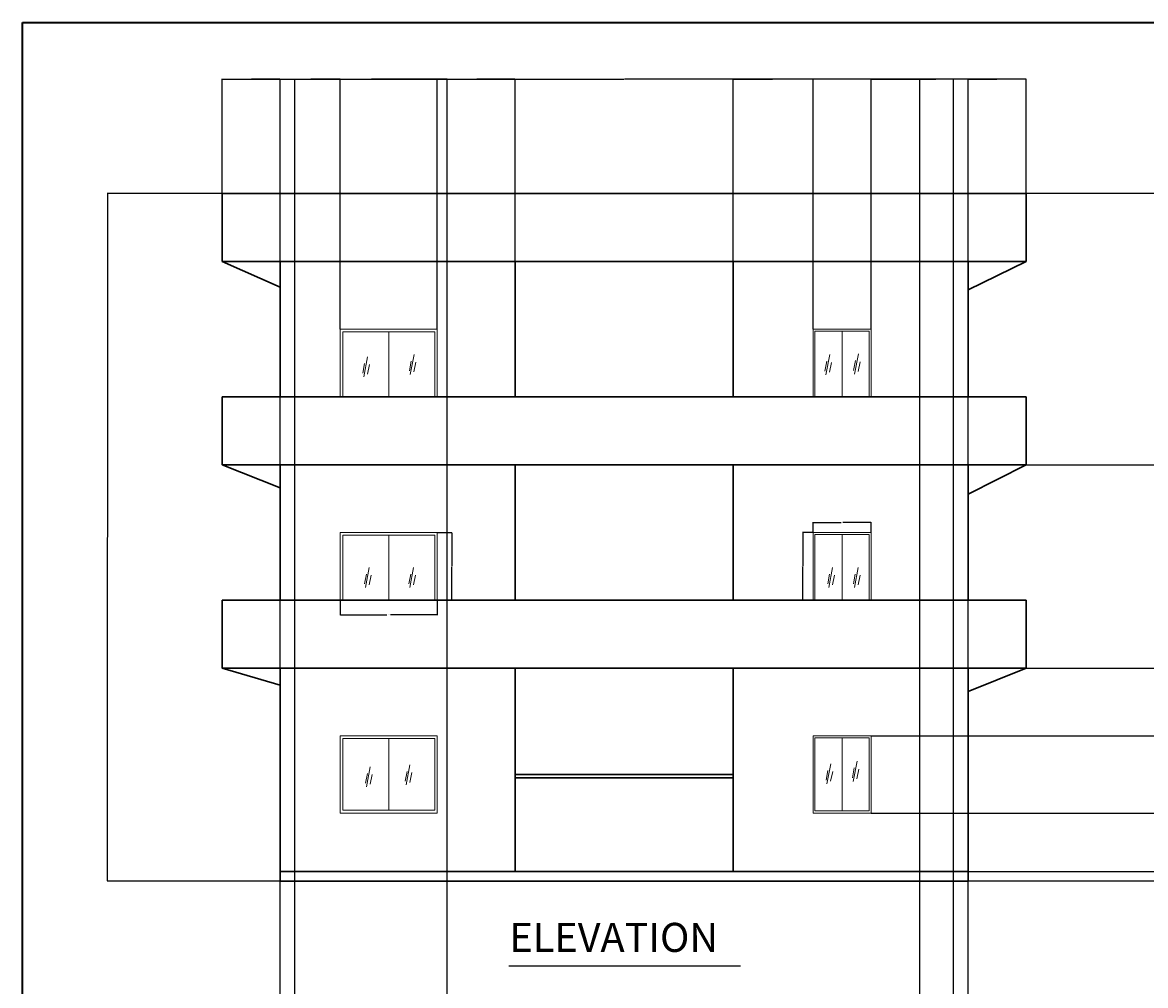
# Model space of a CAD drawing. Units: inches. Extents: x 1355 to 2746, y 1171 to 2751.
# Tile 19 of 24: x 1355 to 2051, y 2155 to 2751. Entities that reach past the tile are written whole.
import ezdxf

# ---------------------------------------------------------------- set-up
doc = ezdxf.new("R2010")
doc.units = ezdxf.units.IN
for name, color, linetype, lineweight in [('A-ANNO-DIMS', 2, 'Continuous', 18), ('A-ANNO-TITL', 7, 'Continuous', 25), ('A-ANNO-TTLB', 7, 'Continuous', 35), ('A-ELEV', 7, 'Continuous', 30), ('A-ELEV-GLAZ', 4, 'Continuous', 18), ('A-WALL-PATT', 252, 'Continuous', 13)]:
    doc.layers.add(name, color=color, linetype=linetype, lineweight=lineweight)
doc.styles.get("Standard").update_dxf_attribs({"font": 'arial.ttf'})
doc.dimstyles.get("Standard").update_dxf_attribs({"dimtxt": 0.18, "dimasz": 0.18, "dimexe": 0.18, "dimexo": 0.0625, "dimgap": 0.09, "dimtad": 0, "dimtih": 1, "dimtoh": 1, "dimdec": 4, "dimzin": 0, "dimdsep": 46, "dimtxsty": 'Standard', "dimcen": 0.09, "dimadec": 0, "dimazin": 0, "dimtfac": 1, "dimtdec": 4, "dimtofl": 0, "dimtmove": 0, "dimatfit": 3, "dimfxl": 1, "dimtolj": 1, "dimtzin": 0, "dimarcsym": 0})

# ---------------------------------------------------------------- blocks, each defined once
blk = doc.blocks.new('WINDOW-ELEV-60')
for p, q in [((0, 42), (0, 0)), ((60, 42), (0, 42)), ((0, 42), (0, 0)), ((60, 42), (0, 42)), ((60, 42), (60, 0)), ((60, 42), (60, 0)), ((30.06, 40.4), (30.06, 0))]:
    blk.add_line(p, q)
blk.add_lwpolyline([(1.53, 0), (1.53, 40.4), (58.59, 40.4), (58.59, 0)])
blk = doc.blocks.new('WINDOW-ELEV-36')
for p, q in [((0, 42), (0, 0)), ((36, 42), (0, 42)), ((0, 42), (0, 0)), ((36, 42), (0, 42)), ((36, 42), (36, 0)), ((36, 42), (36, 0)), ((17.99, 0), (17.99, 40.76))]:
    blk.add_line(p, q)
blk.add_lwpolyline([(1.16, 0), (1.16, 40.76), (34.82, 40.76), (34.82, 0)])
blk = doc.blocks.new('GLASS-REFLECTION')
for p, q in [((1.11, 8.29), (0, 2.25)), ((2.94, 12.42), (0.56, 0)), ((4.09, 7.61), (2.83, 1.61))]:
    blk.add_line(p, q)
blk = doc.blocks.new('*D85')
at = {"layer": 'A-ANNO-DIMS', "color": 0, "lineweight": -2, "transparency": 16777216}
for p, q in [((1551.93, 2393.34), (1551.93, 2384.22)), ((1611.93, 2393.34), (1611.93, 2384.22)), ((1552.11, 2384.4), (1580.82, 2384.4)), ((1611.75, 2384.4), (1583.05, 2384.4))]:
    blk.add_line(p, q, dxfattribs=at)
at = {"layer": 'A-ANNO-DIMS', "color": 0, "transparency": 16777216}
for points in [[(1552.11, 2384.43), (1552.11, 2384.37), (1551.93, 2384.4)], [(1611.75, 2384.43), (1611.75, 2384.37), (1611.93, 2384.4)]]:
    blk.add_solid(points, dxfattribs=at)
at = {"layer": 'Defpoints', "color": 0, "transparency": 16777216}
for p in [(1551.93, 2393.4), (1611.93, 2393.4), (1611.93, 2384.4)]:
    blk.add_point(p, dxfattribs=at)
at = {"layer": 'A-ANNO-DIMS', "color": 0, "transparency": 16777216, "insert": (1581.93, 2384.4), "char_height": 0.18, "attachment_point": 5}
blk.add_mtext('\\A1;WINDOW 60 TYP.', dxfattribs=at)
blk = doc.blocks.new('*D86')
at = {"layer": 'A-ANNO-DIMS', "color": 0, "lineweight": -2, "transparency": 16777216}
for p, q in [((1612, 2435.4), (1621.11, 2435.4)), ((1620.93, 2435.22), (1620.93, 2414.58)), ((1620.93, 2393.58), (1620.93, 2414.22)), ((1612, 2393.4), (1621.11, 2393.4))]:
    blk.add_line(p, q, dxfattribs=at)
at = {"layer": 'A-ANNO-DIMS', "color": 0, "transparency": 16777216}
for points in [[(1620.9, 2435.22), (1620.96, 2435.22), (1620.93, 2435.4)], [(1620.9, 2393.58), (1620.96, 2393.58), (1620.93, 2393.4)]]:
    blk.add_solid(points, dxfattribs=at)
at = {"layer": 'Defpoints', "color": 0, "transparency": 16777216}
for p in [(1611.93, 2435.4), (1620.93, 2435.4), (1611.93, 2393.4)]:
    blk.add_point(p, dxfattribs=at)
at = {"layer": 'A-ANNO-DIMS', "color": 0, "transparency": 16777216, "insert": (1620.93, 2414.4), "char_height": 0.18, "attachment_point": 5}
blk.add_mtext('\\A1;42 TYP.', dxfattribs=at)
blk = doc.blocks.new('*D87')
at = {"layer": 'A-ANNO-DIMS', "color": 0, "lineweight": -2, "transparency": 16777216}
for p, q in [((1844.65, 2435.4), (1838.23, 2435.4)), ((1838.41, 2435.22), (1838.41, 2414.58)), ((1838.41, 2393.58), (1838.41, 2414.22)), ((1844.65, 2393.4), (1838.23, 2393.4))]:
    blk.add_line(p, q, dxfattribs=at)
at = {"layer": 'A-ANNO-DIMS', "color": 0, "transparency": 16777216}
for points in [[(1838.38, 2435.22), (1838.44, 2435.22), (1838.41, 2435.4)], [(1838.38, 2393.58), (1838.44, 2393.58), (1838.41, 2393.4)]]:
    blk.add_solid(points, dxfattribs=at)
at = {"layer": 'Defpoints', "color": 0, "transparency": 16777216}
for p in [(1838.41, 2435.4), (1844.71, 2435.4), (1844.71, 2393.4)]:
    blk.add_point(p, dxfattribs=at)
at = {"layer": 'A-ANNO-DIMS', "color": 0, "transparency": 16777216, "insert": (1838.41, 2414.4), "char_height": 0.18, "attachment_point": 5}
blk.add_mtext('\\A1;WIN. 42 TYP.', dxfattribs=at)
blk = doc.blocks.new('*D88')
at = {"layer": 'A-ANNO-DIMS', "color": 0, "lineweight": -2, "transparency": 16777216}
for p, q in [((1844.71, 2435.46), (1844.71, 2441.88)), ((1844.89, 2441.7), (1862.18, 2441.7)), ((1880.53, 2441.7), (1863.24, 2441.7)), ((1880.71, 2435.46), (1880.71, 2441.88))]:
    blk.add_line(p, q, dxfattribs=at)
at = {"layer": 'A-ANNO-DIMS', "color": 0, "transparency": 16777216}
for points in [[(1844.89, 2441.73), (1844.89, 2441.67), (1844.71, 2441.7)], [(1880.53, 2441.73), (1880.53, 2441.67), (1880.71, 2441.7)]]:
    blk.add_solid(points, dxfattribs=at)
at = {"layer": 'Defpoints', "color": 0, "transparency": 16777216}
for p in [(1880.71, 2441.7), (1844.71, 2435.4), (1880.71, 2435.4)]:
    blk.add_point(p, dxfattribs=at)
at = {"layer": 'A-ANNO-DIMS', "color": 0, "transparency": 16777216, "insert": (1862.71, 2441.7), "char_height": 0.18, "attachment_point": 5}
blk.add_mtext('\\A1;36 TYP.', dxfattribs=at)
blk = doc.blocks.new('*D95')
at = {"layer": 'A-ANNO-DIMS', "color": 0, "lineweight": -2, "transparency": 16777216}
for p, q in [((1514.71, 2139.36), (1514.71, 2716.58)), ((1514.89, 2716.4), (1727.42, 2716.4)), ((1940.53, 2716.4), (1728, 2716.4)), ((1940.71, 2139.36), (1940.71, 2716.58))]:
    blk.add_line(p, q, dxfattribs=at)
at = {"layer": 'A-ANNO-DIMS', "color": 0, "transparency": 16777216}
for points in [[(1514.89, 2716.43), (1514.89, 2716.37), (1514.71, 2716.4)], [(1940.53, 2716.43), (1940.53, 2716.37), (1940.71, 2716.4)]]:
    blk.add_solid(points, dxfattribs=at)
at = {"layer": 'Defpoints', "color": 0, "transparency": 16777216}
for p in [(1940.71, 2716.4), (1514.71, 2139.3), (1940.71, 2139.3)]:
    blk.add_point(p, dxfattribs=at)
at = {"layer": 'A-ANNO-DIMS', "color": 0, "transparency": 16777216, "insert": (1727.71, 2716.4), "char_height": 0.18, "attachment_point": 5}
blk.add_mtext('\\A1;426', dxfattribs=at)
blk = doc.blocks.new('*D114')
at = {"layer": 'A-ANNO-DIMS', "color": 0, "lineweight": -2, "transparency": 16777216}
for p, q in [((1478.71, 2645.46), (1478.71, 2716.58)), ((1478.89, 2716.4), (1727.42, 2716.4)), ((1976.53, 2716.4), (1728, 2716.4)), ((1976.71, 2645.46), (1976.71, 2716.58))]:
    blk.add_line(p, q, dxfattribs=at)
at = {"layer": 'A-ANNO-DIMS', "color": 0, "transparency": 16777216}
for points in [[(1478.89, 2716.43), (1478.89, 2716.37), (1478.71, 2716.4)], [(1976.53, 2716.43), (1976.53, 2716.37), (1976.71, 2716.4)]]:
    blk.add_solid(points, dxfattribs=at)
at = {"layer": 'Defpoints', "color": 0, "transparency": 16777216}
for p in [(1976.71, 2716.4), (1478.71, 2645.4), (1976.71, 2645.4)]:
    blk.add_point(p, dxfattribs=at)
at = {"layer": 'A-ANNO-DIMS', "color": 0, "transparency": 16777216, "insert": (1727.71, 2716.4), "char_height": 0.18, "attachment_point": 5}
blk.add_mtext('\\A1;498', dxfattribs=at)
blk = doc.blocks.new('*D115')
at = {"layer": 'A-ANNO-DIMS', "color": 0, "lineweight": -2, "transparency": 16777216}
for p, q in [((1478.65, 2645.4), (1407.53, 2645.4)), ((1407.71, 2645.22), (1407.71, 2432.58)), ((1407.71, 2219.58), (1407.71, 2432.22)), ((1514.65, 2219.4), (1407.53, 2219.4))]:
    blk.add_line(p, q, dxfattribs=at)
at = {"layer": 'A-ANNO-DIMS', "color": 0, "transparency": 16777216}
for points in [[(1407.68, 2645.22), (1407.74, 2645.22), (1407.71, 2645.4)], [(1407.68, 2219.58), (1407.74, 2219.58), (1407.71, 2219.4)]]:
    blk.add_solid(points, dxfattribs=at)
at = {"layer": 'Defpoints', "color": 0, "transparency": 16777216}
for p in [(1407.71, 2645.4), (1478.71, 2645.4), (1514.71, 2219.4)]:
    blk.add_point(p, dxfattribs=at)
at = {"layer": 'A-ANNO-DIMS', "color": 0, "transparency": 16777216, "insert": (1407.71, 2432.4), "char_height": 0.18, "attachment_point": 5}
blk.add_mtext('\\A1;426', dxfattribs=at)
blk = doc.blocks.new('*D116')
at = {"layer": 'A-ANNO-DIMS', "color": 0, "lineweight": -2, "transparency": 16777216}
for p, q in [((1976.77, 2477.4), (2648.07, 2477.4)), ((2647.89, 2477.22), (2647.89, 2414.58)), ((2647.89, 2351.58), (2647.89, 2414.22)), ((1976.77, 2351.4), (2648.07, 2351.4))]:
    blk.add_line(p, q, dxfattribs=at)
at = {"layer": 'A-ANNO-DIMS', "color": 0, "transparency": 16777216}
for points in [[(2647.86, 2477.22), (2647.92, 2477.22), (2647.89, 2477.4)], [(2647.86, 2351.58), (2647.92, 2351.58), (2647.89, 2351.4)]]:
    blk.add_solid(points, dxfattribs=at)
at = {"layer": 'Defpoints', "color": 0, "transparency": 16777216}
for p in [(1976.71, 2477.4), (2647.89, 2477.4), (1976.71, 2351.4)]:
    blk.add_point(p, dxfattribs=at)
at = {"layer": 'A-ANNO-DIMS', "color": 0, "transparency": 16777216, "insert": (2647.89, 2414.4), "char_height": 0.18, "attachment_point": 5}
blk.add_mtext('\\A1;126', dxfattribs=at)
blk = doc.blocks.new('*D117')
at = {"layer": 'A-ANNO-DIMS', "color": 0, "lineweight": -2, "transparency": 16777216}
for p, q in [((1478.71, 2603.46), (1478.71, 2716.58)), ((1478.89, 2716.4), (1496.49, 2716.4)), ((1514.53, 2716.4), (1496.93, 2716.4)), ((1514.71, 2603.46), (1514.71, 2716.58))]:
    blk.add_line(p, q, dxfattribs=at)
at = {"layer": 'A-ANNO-DIMS', "color": 0, "transparency": 16777216}
for points in [[(1478.89, 2716.43), (1478.89, 2716.37), (1478.71, 2716.4)], [(1514.53, 2716.43), (1514.53, 2716.37), (1514.71, 2716.4)]]:
    blk.add_solid(points, dxfattribs=at)
at = {"layer": 'Defpoints', "color": 0, "transparency": 16777216}
for p in [(1514.71, 2716.4), (1478.71, 2603.4), (1514.71, 2603.4)]:
    blk.add_point(p, dxfattribs=at)
at = {"layer": 'A-ANNO-DIMS', "color": 0, "transparency": 16777216, "insert": (1496.71, 2716.4), "char_height": 0.18, "attachment_point": 5}
blk.add_mtext('\\A1;36', dxfattribs=at)
blk = doc.blocks.new('*D118')
at = {"layer": 'A-ANNO-DIMS', "color": 0, "lineweight": -2, "transparency": 16777216}
for p, q in [((1514.71, 2603.46), (1514.71, 2716.58)), ((1514.89, 2716.4), (1532.86, 2716.4)), ((1551.75, 2716.4), (1533.78, 2716.4)), ((1551.93, 2561.46), (1551.93, 2716.58))]:
    blk.add_line(p, q, dxfattribs=at)
at = {"layer": 'A-ANNO-DIMS', "color": 0, "transparency": 16777216}
for points in [[(1514.89, 2716.43), (1514.89, 2716.37), (1514.71, 2716.4)], [(1551.75, 2716.43), (1551.75, 2716.37), (1551.93, 2716.4)]]:
    blk.add_solid(points, dxfattribs=at)
at = {"layer": 'Defpoints', "color": 0, "transparency": 16777216}
for p in [(1551.93, 2716.4), (1514.71, 2603.4), (1551.93, 2561.4)]:
    blk.add_point(p, dxfattribs=at)
at = {"layer": 'A-ANNO-DIMS', "color": 0, "transparency": 16777216, "insert": (1533.32, 2716.4), "char_height": 0.18, "attachment_point": 5}
blk.add_mtext('\\A1;37.226', dxfattribs=at)
blk = doc.blocks.new('*D119')
at = {"layer": 'A-ANNO-DIMS', "color": 0, "lineweight": -2, "transparency": 16777216}
for p, q in [((1611.93, 2561.46), (1611.93, 2716.58)), ((1612.11, 2716.4), (1635.67, 2716.4)), ((1660.03, 2716.4), (1636.47, 2716.4)), ((1660.21, 2603.46), (1660.21, 2716.58))]:
    blk.add_line(p, q, dxfattribs=at)
at = {"layer": 'A-ANNO-DIMS', "color": 0, "transparency": 16777216}
for points in [[(1612.11, 2716.43), (1612.11, 2716.37), (1611.93, 2716.4)], [(1660.03, 2716.43), (1660.03, 2716.37), (1660.21, 2716.4)]]:
    blk.add_solid(points, dxfattribs=at)
at = {"layer": 'Defpoints', "color": 0, "transparency": 16777216}
for p in [(1660.21, 2716.4), (1660.21, 2603.4), (1611.93, 2561.4)]:
    blk.add_point(p, dxfattribs=at)
at = {"layer": 'A-ANNO-DIMS', "color": 0, "transparency": 16777216, "insert": (1636.07, 2716.4), "char_height": 0.18, "attachment_point": 5}
blk.add_mtext('\\A1;48.27', dxfattribs=at)
blk = doc.blocks.new('*D120')
at = {"layer": 'A-ANNO-DIMS', "color": 0, "lineweight": -2, "transparency": 16777216}
for p, q in [((1660.21, 2603.46), (1660.21, 2716.58)), ((1660.39, 2716.4), (1727.43, 2716.4)), ((1795.03, 2716.4), (1727.99, 2716.4)), ((1795.21, 2603.46), (1795.21, 2716.58))]:
    blk.add_line(p, q, dxfattribs=at)
at = {"layer": 'A-ANNO-DIMS', "color": 0, "transparency": 16777216}
for points in [[(1660.39, 2716.43), (1660.39, 2716.37), (1660.21, 2716.4)], [(1795.03, 2716.43), (1795.03, 2716.37), (1795.21, 2716.4)]]:
    blk.add_solid(points, dxfattribs=at)
at = {"layer": 'Defpoints', "color": 0, "transparency": 16777216}
for p in [(1795.21, 2716.4), (1660.21, 2603.4), (1795.21, 2603.4)]:
    blk.add_point(p, dxfattribs=at)
at = {"layer": 'A-ANNO-DIMS', "color": 0, "transparency": 16777216, "insert": (1727.71, 2716.4), "char_height": 0.18, "attachment_point": 5}
blk.add_mtext('\\A1;135', dxfattribs=at)
blk = doc.blocks.new('*D121')
at = {"layer": 'A-ANNO-DIMS', "color": 0, "lineweight": -2, "transparency": 16777216}
for p, q in [((1795.21, 2603.46), (1795.21, 2716.58)), ((1795.39, 2716.4), (1819.63, 2716.4)), ((1844.53, 2716.4), (1820.29, 2716.4)), ((1844.71, 2561.46), (1844.71, 2716.58))]:
    blk.add_line(p, q, dxfattribs=at)
at = {"layer": 'A-ANNO-DIMS', "color": 0, "transparency": 16777216}
for points in [[(1795.39, 2716.43), (1795.39, 2716.37), (1795.21, 2716.4)], [(1844.53, 2716.43), (1844.53, 2716.37), (1844.71, 2716.4)]]:
    blk.add_solid(points, dxfattribs=at)
at = {"layer": 'Defpoints', "color": 0, "transparency": 16777216}
for p in [(1844.71, 2716.4), (1795.21, 2603.4), (1844.71, 2561.4)]:
    blk.add_point(p, dxfattribs=at)
at = {"layer": 'A-ANNO-DIMS', "color": 0, "transparency": 16777216, "insert": (1819.96, 2716.4), "char_height": 0.18, "attachment_point": 5}
blk.add_mtext('\\A1;49.5', dxfattribs=at)
blk = doc.blocks.new('*D122')
at = {"layer": 'A-ANNO-DIMS', "color": 0, "lineweight": -2, "transparency": 16777216}
for p, q in [((1880.71, 2561.46), (1880.71, 2716.58)), ((1880.89, 2716.4), (1910.49, 2716.4)), ((1940.53, 2716.4), (1910.93, 2716.4)), ((1940.71, 2603.46), (1940.71, 2716.58))]:
    blk.add_line(p, q, dxfattribs=at)
at = {"layer": 'A-ANNO-DIMS', "color": 0, "transparency": 16777216}
for points in [[(1880.89, 2716.43), (1880.89, 2716.37), (1880.71, 2716.4)], [(1940.53, 2716.43), (1940.53, 2716.37), (1940.71, 2716.4)]]:
    blk.add_solid(points, dxfattribs=at)
at = {"layer": 'Defpoints', "color": 0, "transparency": 16777216}
for p in [(1940.71, 2716.4), (1940.71, 2603.4), (1880.71, 2561.4)]:
    blk.add_point(p, dxfattribs=at)
at = {"layer": 'A-ANNO-DIMS', "color": 0, "transparency": 16777216, "insert": (1910.71, 2716.4), "char_height": 0.18, "attachment_point": 5}
blk.add_mtext('\\A1;60', dxfattribs=at)
blk = doc.blocks.new('*D123')
at = {"layer": 'A-ANNO-DIMS', "color": 0, "lineweight": -2, "transparency": 16777216}
for p, q in [((1880.77, 2261.4), (2648.07, 2261.4)), ((2647.89, 2261.22), (2647.89, 2243.58)), ((2647.89, 2225.58), (2647.89, 2243.22)), ((1940.77, 2225.4), (2648.07, 2225.4))]:
    blk.add_line(p, q, dxfattribs=at)
at = {"layer": 'A-ANNO-DIMS', "color": 0, "transparency": 16777216}
for points in [[(2647.86, 2261.22), (2647.92, 2261.22), (2647.89, 2261.4)], [(2647.86, 2225.58), (2647.92, 2225.58), (2647.89, 2225.4)]]:
    blk.add_solid(points, dxfattribs=at)
at = {"layer": 'Defpoints', "color": 0, "transparency": 16777216}
for p in [(1880.71, 2261.4), (2647.89, 2261.4), (1940.71, 2225.4)]:
    blk.add_point(p, dxfattribs=at)
at = {"layer": 'A-ANNO-DIMS', "color": 0, "transparency": 16777216, "insert": (2647.89, 2243.4), "char_height": 0.18, "attachment_point": 5}
blk.add_mtext('\\A1;36', dxfattribs=at)
blk = doc.blocks.new('*D124')
at = {"layer": 'A-ANNO-DIMS', "color": 0, "lineweight": -2, "transparency": 16777216}
for p, q in [((1940.71, 2603.46), (1940.71, 2716.58)), ((1940.89, 2716.4), (1958.49, 2716.4)), ((1976.53, 2716.4), (1958.93, 2716.4)), ((1976.71, 2603.46), (1976.71, 2716.58))]:
    blk.add_line(p, q, dxfattribs=at)
at = {"layer": 'A-ANNO-DIMS', "color": 0, "transparency": 16777216}
for points in [[(1940.89, 2716.43), (1940.89, 2716.37), (1940.71, 2716.4)], [(1976.53, 2716.43), (1976.53, 2716.37), (1976.71, 2716.4)]]:
    blk.add_solid(points, dxfattribs=at)
at = {"layer": 'Defpoints', "color": 0, "transparency": 16777216}
for p in [(1976.71, 2716.4), (1940.71, 2603.4), (1976.71, 2603.4)]:
    blk.add_point(p, dxfattribs=at)
at = {"layer": 'A-ANNO-DIMS', "color": 0, "transparency": 16777216, "insert": (1958.71, 2716.4), "char_height": 0.18, "attachment_point": 5}
blk.add_mtext('\\A1;36', dxfattribs=at)
blk = doc.blocks.new('*D125')
at = {"layer": 'A-ANNO-DIMS', "color": 0, "lineweight": -2, "transparency": 16777216}
for p, q in [((1880.77, 2309.4), (2648.07, 2309.4)), ((2647.89, 2309.22), (2647.89, 2285.58)), ((2647.89, 2261.58), (2647.89, 2285.22)), ((1880.77, 2261.4), (2648.07, 2261.4))]:
    blk.add_line(p, q, dxfattribs=at)
at = {"layer": 'A-ANNO-DIMS', "color": 0, "transparency": 16777216}
for points in [[(2647.86, 2309.22), (2647.92, 2309.22), (2647.89, 2309.4)], [(2647.86, 2261.58), (2647.92, 2261.58), (2647.89, 2261.4)]]:
    blk.add_solid(points, dxfattribs=at)
at = {"layer": 'Defpoints', "color": 0, "transparency": 16777216}
for p in [(1880.71, 2309.4), (2647.89, 2309.4), (1880.71, 2261.4)]:
    blk.add_point(p, dxfattribs=at)
at = {"layer": 'A-ANNO-DIMS', "color": 0, "transparency": 16777216, "insert": (2647.89, 2285.4), "char_height": 0.18, "attachment_point": 5}
blk.add_mtext('\\A1;48', dxfattribs=at)
blk = doc.blocks.new('*D127')
at = {"layer": 'A-ANNO-DIMS', "color": 0, "lineweight": -2, "transparency": 16777216}
for p, q in [((2080.33, 2645.4), (1407.53, 2645.4)), ((1407.71, 2645.22), (1407.71, 2432.58)), ((1407.71, 2219.58), (1407.71, 2432.22)), ((2080.33, 2219.4), (1407.53, 2219.4))]:
    blk.add_line(p, q, dxfattribs=at)
at = {"layer": 'A-ANNO-DIMS', "color": 0, "transparency": 16777216}
for points in [[(1407.68, 2645.22), (1407.74, 2645.22), (1407.71, 2645.4)], [(1407.68, 2219.58), (1407.74, 2219.58), (1407.71, 2219.4)]]:
    blk.add_solid(points, dxfattribs=at)
at = {"layer": 'Defpoints', "color": 0, "transparency": 16777216}
for p in [(1407.71, 2645.4), (2080.39, 2645.4), (2080.39, 2219.4)]:
    blk.add_point(p, dxfattribs=at)
at = {"layer": 'A-ANNO-DIMS', "color": 0, "transparency": 16777216, "insert": (1407.71, 2432.4), "char_height": 0.18, "attachment_point": 5}
blk.add_mtext('\\A1;426', dxfattribs=at)
blk = doc.blocks.new('*D135')
at = {"layer": 'A-ANNO-DIMS', "color": 0, "lineweight": -2, "transparency": 16777216}
for p, q in [((1523.71, 1981.86), (1523.71, 2716.58)), ((1523.89, 2716.4), (1570.63, 2716.4)), ((1618.03, 2716.4), (1571.28, 2716.4)), ((1618.21, 1981.86), (1618.21, 2716.58))]:
    blk.add_line(p, q, dxfattribs=at)
at = {"layer": 'A-ANNO-DIMS', "color": 0, "transparency": 16777216}
for points in [[(1523.89, 2716.43), (1523.89, 2716.37), (1523.71, 2716.4)], [(1618.03, 2716.43), (1618.03, 2716.37), (1618.21, 2716.4)]]:
    blk.add_solid(points, dxfattribs=at)
at = {"layer": 'Defpoints', "color": 0, "transparency": 16777216}
for p in [(1618.21, 2716.4), (1523.71, 1981.8), (1618.21, 1981.8)]:
    blk.add_point(p, dxfattribs=at)
at = {"layer": 'A-ANNO-DIMS', "color": 0, "transparency": 16777216, "insert": (1570.96, 2716.4), "char_height": 0.18, "attachment_point": 5}
blk.add_mtext('\\A1;94.5', dxfattribs=at)
blk = doc.blocks.new('*D145')
at = {"layer": 'A-ANNO-DIMS', "color": 0, "lineweight": -2, "transparency": 16777216}
for p, q in [((1910.88, 1399.86), (1910.88, 2716.58)), ((1911.06, 2716.4), (1920.83, 2716.4)), ((1931.53, 2716.4), (1921.76, 2716.4)), ((1931.71, 1399.86), (1931.71, 2716.58))]:
    blk.add_line(p, q, dxfattribs=at)
at = {"layer": 'A-ANNO-DIMS', "color": 0, "transparency": 16777216}
for points in [[(1911.06, 2716.43), (1911.06, 2716.37), (1910.88, 2716.4)], [(1931.53, 2716.43), (1931.53, 2716.37), (1931.71, 2716.4)]]:
    blk.add_solid(points, dxfattribs=at)
at = {"layer": 'Defpoints', "color": 0, "transparency": 16777216}
for p in [(1931.71, 2716.4), (1910.88, 1399.8), (1931.71, 1399.8)]:
    blk.add_point(p, dxfattribs=at)
at = {"layer": 'A-ANNO-DIMS', "color": 0, "transparency": 16777216, "insert": (1921.3, 2716.4), "char_height": 0.18, "attachment_point": 5}
blk.add_mtext('\\A1;20.824', dxfattribs=at)

msp = doc.modelspace()

# ---------------------------------------------------------------- hatches: boundary and pattern name
at = {"layer": 'A-WALL-PATT'}
h = msp.add_hatch(dxfattribs=at)
h.set_pattern_fill('ANSI32', color=256)
h.paths.add_polyline_path([(1660.2083, 2139.3018), (1614.5977, 2139.3018), (1614.5977, 2130.3018), (1655.7083, 2130.3018), (1655.7083, 1981.8018), (1660.2083, 1981.8018), (1660.2083, 2090.7225), (1692.5832, 2090.7225), (1692.5832, 2095.2225), (1660.2083, 2095.2225)])
h.paths.add_polyline_path([(1523.7083, 2130.3018), (1554.5977, 2130.3018), (1554.5977, 2134.8018), (1554.5977, 2139.3018), (1514.7083, 2139.3018), (1514.7083, 2071.8385), (1523.7083, 2071.8385)])
h.paths.add_polyline_path([(1940.7083, 2139.3018), (1883.7928, 2139.3018), (1883.7928, 2130.3018), (1931.7083, 2130.3018), (1931.7083, 2098.3333), (1940.7083, 2098.3333)])
h.paths.add_polyline_path([(1799.7083, 2130.3018), (1823.7928, 2130.3018), (1823.7928, 2134.8018), (1823.7928, 2139.3018), (1795.2083, 2139.3018), (1795.2083, 2130.3018), (1795.2083, 2095.2225), (1759.2134, 2095.2225), (1759.2134, 2090.7225), (1795.2083, 2090.7225), (1795.2083, 1981.8018), (1799.7083, 1981.8018), (1799.7083, 1986.3018)])
h.paths.add_polyline_path([(1940.7083, 2038.3333), (1931.7083, 2038.3333), (1931.7083, 1986.3018), (1832.7083, 1986.3018), (1832.7083, 1947.1338), (1837.2083, 1947.1338), (1837.2083, 1981.8018), (1931.7083, 1981.8018), (1931.7083, 1967.1939), (1940.7083, 1967.1939)])
h.paths.add_polyline_path([(1940.7083, 1943.1939), (1931.7083, 1943.1939), (1931.7083, 1921.8018), (1837.2083, 1921.8018), (1837.2083, 1926.0511), (1832.7083, 1926.0511), (1832.7083, 1917.3018), (1931.7083, 1917.3018), (1931.7083, 1908.3321), (1940.7083, 1908.3321)])
h.paths.add_polyline_path([(1940.7083, 1884.3321), (1931.7083, 1884.3321), (1931.7083, 1869.3018), (1899.4583, 1869.3018), (1899.4583, 1864.8018), (1931.7083, 1864.8018), (1931.7083, 1773.3018), (1786.5143, 1773.3018), (1786.5143, 1764.3018), (1844.7083, 1764.3018), (1844.7083, 1748.9343), (1853.7083, 1748.9343), (1853.7083, 1764.3018), (1931.7083, 1764.3018), (1931.7083, 1652.9424), (1940.7083, 1652.9424)])
h.paths.add_polyline_path([(1799.7083, 1864.8018), (1806.0522, 1864.8018), (1806.0522, 1867.0518), (1806.0522, 1869.3018), (1799.7083, 1869.3018), (1799.7083, 1917.3018), (1799.7083, 1921.8018), (1795.2083, 1921.8018), (1795.2083, 1773.3018), (1799.7083, 1773.3018)])
h.paths.add_polyline_path([(1872.8988, 1867.0518), (1872.8988, 1869.3018), (1867.2083, 1869.3018), (1867.2083, 1917.3018), (1862.7083, 1917.3018), (1862.7083, 1869.3018), (1836.9546, 1869.3018), (1836.9546, 1864.8018), (1862.7083, 1864.8018), (1872.8988, 1864.8018)])
h.paths.add_polyline_path([(1749.2197, 1773.3018), (1655.7083, 1773.3018), (1523.7083, 1773.3018), (1523.7083, 1828.4963), (1514.7083, 1828.4963), (1514.7083, 1753.9033), (1519.2083, 1753.9033), (1523.7083, 1753.9033), (1523.7083, 1764.3018), (1655.7083, 1764.3018), (1749.2197, 1764.3018), (1749.2197, 1768.8018)])
h.paths.add_polyline_path([(1660.2083, 1921.8018), (1655.7083, 1921.8018), (1655.7083, 1917.3018), (1655.7083, 1773.3018), (1660.2083, 1773.3018)])
h.paths.add_polyline_path([(1523.7083, 2011.8385), (1514.7083, 2011.8385), (1514.7083, 1973.114), (1519.2083, 1973.114), (1523.7083, 1973.114), (1523.7083, 1976.8227), (1523.7083, 1981.8018), (1618.2083, 1981.8018), (1618.2083, 1921.8018), (1553.707, 1921.8018), (1553.707, 1917.3018), (1622.7083, 1917.3018), (1622.7083, 1919.5518), (1622.7083, 1921.8018), (1622.7083, 1986.3018), (1523.7083, 1986.3018)])
h.paths.add_polyline_path([(1529.6686, 1919.5518), (1529.6686, 1921.8018), (1523.7083, 1921.8018), (1523.7083, 1949.114), (1514.7083, 1949.114), (1514.7083, 1888.4963), (1523.7083, 1888.4963), (1523.7083, 1917.3018), (1529.6686, 1917.3018)])
h.paths.add_polyline_path([(1538.9419, 1775.643), (1585.5504, 1775.643), (1585.5504, 1798.0318), (1538.9419, 1798.0318)], flags=25)
h.paths.add_polyline_path([(1696.7097, 1497.3356), (1769.5651, 1497.3356), (1769.5651, 1523.4559), (1696.7097, 1523.4559)], flags=9)
h.paths.add_polyline_path([(1629.1643, 1230.5133), (1877.0879, 1230.5133), (1877.0879, 1267.606), (1629.1643, 1267.606)], flags=9)
h.paths.add_polyline_path([(2533.4462, 2215.4033), (2579.9292, 2215.4033), (2579.9292, 2231.889), (2533.4462, 2231.889)], flags=9)
h.paths.add_polyline_path([(2540.822, 2515.6945), (2594.2245, 2515.6945), (2594.2245, 2545.5463), (2540.822, 2545.5463)], flags=9)
h.paths.add_polyline_path([(2535.9857, 2588.2819), (2582.4687, 2588.2819), (2582.4687, 2604.7675), (2535.9857, 2604.7675)], flags=9)
h.paths.add_polyline_path([(2537.1627, 2617.1172), (2649.1245, 2617.1172), (2649.1245, 2633.6029), (2537.1627, 2633.6029)], flags=9)
h.paths.add_polyline_path([(2218.0051, 2168.228), (2363.9573, 2168.228), (2363.9573, 2205.3208), (2218.0051, 2205.3208)], flags=9)
h.paths.add_polyline_path([(1650.2156, 2165.3631), (1800.3547, 2165.3631), (1800.3547, 2202.4559), (1650.2156, 2202.4559)], flags=9)
h.paths.add_polyline_path([(2553.9592, 1610.7663), (2588.4203, 1610.7663), (2588.4203, 1660.2233), (2553.9592, 1660.2233)], flags=9)
h.paths.add_polyline_path([(1549.0868, 1648.2033), (1595.6952, 1648.2033), (1595.6952, 1670.5921), (1549.0868, 1670.5921)], flags=9)
h.paths.add_polyline_path([(1546.9525, 1502.0931), (1583.3413, 1502.0931), (1583.3413, 1524.4819), (1546.9525, 1524.4819)], flags=9)
h.paths.add_polyline_path([(1540.7704, 1433.4431), (1587.3788, 1433.4431), (1587.3788, 1455.8319), (1540.7704, 1455.8319)], flags=9)
h.paths.add_polyline_path([(1683.6524, 1321.5269), (1760.6169, 1321.5269), (1760.6169, 1333.8911), (1683.6524, 1333.8911)], flags=9)
h.paths.add_polyline_path([(1832.0485, 1356.0874), (1873.0989, 1356.0874), (1873.0989, 1378.4762), (1832.0485, 1378.4762)], flags=9)
h.paths.add_polyline_path([(1877.9694, 1431.2138), (1926.3827, 1431.2138), (1926.3827, 1453.578), (1877.9694, 1453.578)], flags=9)
h.paths.add_polyline_path([(1847.3106, 1499.8371), (1883.6994, 1499.8371), (1883.6994, 1522.2259), (1847.3106, 1522.2259)], flags=9)
h.paths.add_polyline_path([(1813.7015, 1640.7287), (1860.3099, 1640.7287), (1860.3099, 1663.1175), (1813.7015, 1663.1175)], flags=9)
h.paths.add_polyline_path([(1876.2576, 1710.2471), (1912.9452, 1710.2471), (1912.9452, 1732.6359), (1876.2576, 1732.6359)], flags=25)
h.paths.add_polyline_path([(1695.9163, 1715.3064), (1736.9668, 1715.3064), (1736.9668, 1737.6952), (1695.9163, 1737.6952)], flags=9)
h.paths.add_polyline_path([(1881.8583, 1888.9094), (1930.2717, 1888.9094), (1930.2717, 1911.2737), (1881.8583, 1911.2737)], flags=9)
h.paths.add_polyline_path([(1823.9298, 1798.6431), (1864.9803, 1798.6431), (1864.9803, 1821.0319), (1823.9298, 1821.0319)], flags=25)
h.paths.add_polyline_path([(1845.6062, 1948.1408), (1881.995, 1948.1408), (1881.995, 1970.5296), (1845.6062, 1970.5296)], flags=25)
h.paths.add_polyline_path([(1849.027, 1991.5151), (1895.6355, 1991.5151), (1895.6355, 2013.9039), (1849.027, 2013.9039)], flags=25)
h.paths.add_polyline_path([(1684.9725, 2113.8416), (1764.2658, 2113.8416), (1764.2658, 2126.2058), (1684.9725, 2126.2058)], flags=9)
h.paths.add_polyline_path([(1688.6193, 1913.0676), (1776.2005, 1913.0676), (1776.2005, 1935.4564), (1688.6193, 1935.4564)], flags=9)
h.paths.add_polyline_path([(1571.4689, 1930.9816), (1607.8577, 1930.9816), (1607.8577, 1953.3704), (1571.4689, 1953.3704)], flags=25)
h.paths.add_polyline_path([(1535.3581, 1998.3125), (1581.9665, 1998.3125), (1581.9665, 2020.7014), (1535.3581, 2020.7014)], flags=9)
h = msp.add_hatch(dxfattribs=at)
h.set_pattern_fill('ANSI32', color=256)
h.paths.add_polyline_path([(1749.2197, 1686.3018), (1732.6892, 1686.3018), (1523.7083, 1686.3018), (1523.7083, 1705.9033), (1514.7083, 1705.9033), (1514.7083, 1647.8732), (1519.2083, 1647.8732), (1523.7083, 1647.8732), (1523.7083, 1677.3018), (1655.7083, 1677.3018), (1655.7083, 1528.8018), (1660.2083, 1528.8018), (1660.2083, 1677.3018), (1732.6892, 1677.3018), (1749.2197, 1677.3018)])
h.paths.add_polyline_path([(1931.7083, 1686.3018), (1853.7083, 1686.3018), (1853.7083, 1703.5696), (1844.7083, 1703.5696), (1844.7083, 1686.3018), (1788.0274, 1686.3018), (1788.0274, 1677.3018), (1795.2083, 1677.3018), (1795.2083, 1528.8018), (1799.7083, 1528.8018), (1799.7083, 1677.3018), (1844.7083, 1677.3018), (1931.7083, 1677.3018)])
h.paths.add_polyline_path([(1931.7083, 1533.3018), (1844.7083, 1533.3018), (1832.7083, 1533.3018), (1832.7083, 1531.0518), (1832.7083, 1528.8018), (1832.7083, 1495.7519), (1837.2083, 1495.7519), (1837.2083, 1528.8018), (1931.7083, 1528.8018)])
h.paths.add_polyline_path([(1940.7083, 1592.9424), (1931.7083, 1592.9424), (1931.7083, 1506.7845), (1940.7083, 1506.7845)])
h.paths.add_polyline_path([(1940.7083, 1482.7845), (1936.2083, 1482.7845), (1931.7083, 1482.7845), (1931.7083, 1320.3018), (1880.7083, 1320.3018), (1880.7083, 1311.3018), (1940.7083, 1311.3018)])
h.paths.add_polyline_path([(1931.7083, 1468.8018), (1844.7083, 1468.8018), (1837.2083, 1468.8018), (1837.2083, 1474.34), (1832.7083, 1474.34), (1832.7083, 1468.8018), (1832.7083, 1464.3018), (1844.7083, 1464.3018), (1931.7083, 1464.3018)])
h.paths.add_polyline_path([(1863.8571, 1464.3018), (1859.3571, 1464.3018), (1859.3571, 1404.1662), (1838.1542, 1404.1662), (1838.1542, 1399.8018), (1869.4185, 1399.8018), (1869.4185, 1402.0518), (1869.4185, 1404.3018), (1863.8571, 1404.3018)])
h.paths.add_polyline_path([(1799.7083, 1399.6662), (1805.4082, 1399.6662), (1805.4082, 1401.9162), (1805.4082, 1404.1662), (1799.7083, 1404.1662), (1799.7083, 1464.3018), (1799.7083, 1468.8018), (1795.2083, 1468.8018), (1795.2083, 1356.2098), (1761.2597, 1356.2098), (1761.2597, 1351.7098), (1795.2083, 1351.7098), (1795.2083, 1320.3018), (1795.2083, 1311.3018), (1844.7083, 1311.3018), (1844.7083, 1315.8018), (1844.7083, 1320.3018), (1799.7083, 1320.3018)])
h.paths.add_polyline_path([(1692.9218, 1356.2098), (1660.2083, 1356.2098), (1660.2083, 1430.786), (1657.9583, 1430.786), (1655.7083, 1430.786), (1655.7083, 1320.3018), (1611.934, 1320.3018), (1611.934, 1311.3018), (1660.2083, 1311.3018), (1660.2083, 1351.7098), (1692.9218, 1351.7098)])
h.paths.add_polyline_path([(1523.7083, 1372.653), (1514.7083, 1372.653), (1514.7083, 1311.3018), (1551.934, 1311.3018), (1551.934, 1315.8018), (1551.934, 1320.3018), (1523.7083, 1320.3018)])
h.paths.add_polyline_path([(1523.7083, 1490.9023), (1514.7083, 1490.9023), (1514.7083, 1432.653), (1519.2083, 1432.653), (1523.7083, 1432.653)])
h.paths.add_polyline_path([(1660.2083, 1468.8018), (1622.7083, 1468.8018), (1622.7083, 1473.1566), (1618.2083, 1473.1566), (1618.2083, 1468.8018), (1523.7083, 1468.8018), (1523.7083, 1464.3018), (1655.7083, 1464.3018), (1655.7083, 1460.5634), (1660.2083, 1460.5634)])
h.paths.add_polyline_path([(1523.7083, 1587.8732), (1514.7083, 1587.8732), (1514.7083, 1514.9023), (1519.2083, 1514.9023), (1523.7083, 1514.9023)])
h.paths.add_polyline_path([(1622.7083, 1533.3018), (1523.7083, 1533.3018), (1523.7083, 1528.8018), (1618.2083, 1528.8018), (1618.2083, 1494.4205), (1622.7083, 1494.4205), (1622.7083, 1528.8018)])
h.paths.add_polyline_path([(1696.7097, 1497.3356), (1769.5651, 1497.3356), (1769.5651, 1523.4559), (1696.7097, 1523.4559)], flags=9)
h.paths.add_polyline_path([(1629.1643, 1230.5133), (1877.0879, 1230.5133), (1877.0879, 1267.606), (1629.1643, 1267.606)], flags=9)
h.paths.add_polyline_path([(2533.4462, 2215.4033), (2579.9292, 2215.4033), (2579.9292, 2231.889), (2533.4462, 2231.889)], flags=9)
h.paths.add_polyline_path([(2540.822, 2515.6945), (2594.2245, 2515.6945), (2594.2245, 2545.5463), (2540.822, 2545.5463)], flags=9)
h.paths.add_polyline_path([(2535.9857, 2588.2819), (2582.4687, 2588.2819), (2582.4687, 2604.7675), (2535.9857, 2604.7675)], flags=9)
h.paths.add_polyline_path([(2537.1627, 2617.1172), (2649.1245, 2617.1172), (2649.1245, 2633.6029), (2537.1627, 2633.6029)], flags=9)
h.paths.add_polyline_path([(2218.0051, 2168.228), (2363.9573, 2168.228), (2363.9573, 2205.3208), (2218.0051, 2205.3208)], flags=9)
h.paths.add_polyline_path([(1650.2156, 2165.3631), (1800.3547, 2165.3631), (1800.3547, 2202.4559), (1650.2156, 2202.4559)], flags=9)
h.paths.add_polyline_path([(2553.9592, 1610.7663), (2588.4203, 1610.7663), (2588.4203, 1660.2233), (2553.9592, 1660.2233)], flags=9)
h.paths.add_polyline_path([(1549.0868, 1648.2033), (1595.6952, 1648.2033), (1595.6952, 1670.5921), (1549.0868, 1670.5921)], flags=25)
h.paths.add_polyline_path([(1546.9525, 1502.0931), (1583.3413, 1502.0931), (1583.3413, 1524.4819), (1546.9525, 1524.4819)], flags=25)
h.paths.add_polyline_path([(1540.7704, 1433.4431), (1587.3788, 1433.4431), (1587.3788, 1455.8319), (1540.7704, 1455.8319)], flags=9)
h.paths.add_polyline_path([(1683.6524, 1321.5269), (1760.6169, 1321.5269), (1760.6169, 1333.8911), (1683.6524, 1333.8911)], flags=9)
h.paths.add_polyline_path([(1832.0485, 1356.0874), (1873.0989, 1356.0874), (1873.0989, 1378.4762), (1832.0485, 1378.4762)], flags=9)
h.paths.add_polyline_path([(1877.9694, 1431.2138), (1926.3827, 1431.2138), (1926.3827, 1453.578), (1877.9694, 1453.578)], flags=9)
h.paths.add_polyline_path([(1847.3106, 1499.8371), (1883.6994, 1499.8371), (1883.6994, 1522.2259), (1847.3106, 1522.2259)], flags=25)
h.paths.add_polyline_path([(1813.7015, 1640.7287), (1860.3099, 1640.7287), (1860.3099, 1663.1175), (1813.7015, 1663.1175)], flags=25)
h.paths.add_polyline_path([(1876.2576, 1710.2471), (1912.9452, 1710.2471), (1912.9452, 1732.6359), (1876.2576, 1732.6359)], flags=9)
h.paths.add_polyline_path([(1695.9163, 1715.3064), (1736.9668, 1715.3064), (1736.9668, 1737.6952), (1695.9163, 1737.6952)], flags=9)
h.paths.add_polyline_path([(1881.8583, 1888.9094), (1930.2717, 1888.9094), (1930.2717, 1911.2737), (1881.8583, 1911.2737)], flags=9)
h.paths.add_polyline_path([(1823.9298, 1798.6431), (1864.9803, 1798.6431), (1864.9803, 1821.0319), (1823.9298, 1821.0319)], flags=9)
h.paths.add_polyline_path([(1845.6062, 1948.1408), (1881.995, 1948.1408), (1881.995, 1970.5296), (1845.6062, 1970.5296)], flags=9)
h.paths.add_polyline_path([(1849.027, 1991.5151), (1895.6355, 1991.5151), (1895.6355, 2013.9039), (1849.027, 2013.9039)], flags=9)
h.paths.add_polyline_path([(1684.9725, 2113.8416), (1764.2658, 2113.8416), (1764.2658, 2126.2058), (1684.9725, 2126.2058)], flags=9)
h.paths.add_polyline_path([(1688.6193, 1913.0676), (1776.2005, 1913.0676), (1776.2005, 1935.4564), (1688.6193, 1935.4564)], flags=9)
h.paths.add_polyline_path([(1538.9419, 1775.643), (1585.5504, 1775.643), (1585.5504, 1798.0318), (1538.9419, 1798.0318)], flags=9)
h.paths.add_polyline_path([(1571.4689, 1930.9816), (1607.8577, 1930.9816), (1607.8577, 1953.3704), (1571.4689, 1953.3704)], flags=9)
h.paths.add_polyline_path([(1535.3581, 1998.3125), (1581.9665, 1998.3125), (1581.9665, 2020.7014), (1535.3581, 2020.7014)], flags=9)

# ---------------------------------------------------------------- linework, layer by layer
at = {"layer": 'A-ANNO-TITL'}
msp.add_line((1656.2076, 2166.8872), (1799.8868, 2166.8872), dxfattribs=at)
at = {"layer": 'A-ANNO-TTLB'}
msp.add_lwpolyline([(1355.0901, 2751.4741), (2746.1804, 2751.4741), (2746.1804, 1182.883), (1355.0901, 1182.883)], close=True, dxfattribs=at)
at = {"layer": 'A-ELEV'}
for p, q in [((1976.7083, 2645.3999), (1478.7083, 2645.3999)), ((1478.7083, 2603.3999), (1478.7083, 2645.3999)), ((1976.7083, 2603.3999), (1976.7083, 2645.3999)), ((1976.7083, 2603.3999), (1478.7083, 2603.3999)), ((1478.7083, 2603.3999), (1514.7083, 2587.3654)), ((1514.7083, 2603.3999), (1514.7083, 2519.3999)), ((1660.2083, 2603.3999), (1660.2083, 2519.3999)), ((1795.2083, 2603.3999), (1795.2083, 2519.3999)), ((1940.7083, 2603.3999), (1940.7083, 2519.3999)), ((1976.7083, 2603.3999), (1940.7083, 2585.6865)), ((1660.2083, 2519.3999), (1660.2083, 2537.3999)), ((1795.2083, 2537.3999), (1795.2083, 2535.3999)), ((1976.7083, 2519.3999), (1478.7083, 2519.3999)), ((1478.7083, 2477.3999), (1478.7083, 2519.3999)), ((1976.7083, 2477.3999), (1976.7083, 2519.3999)), ((1976.7083, 2477.3999), (1478.7083, 2477.3999)), ((1478.7083, 2477.3999), (1514.7083, 2463.0175)), ((1514.7083, 2477.3999), (1514.7083, 2393.3999)), ((1514.7083, 2477.3999), (1514.7083, 2471.3999)), ((1660.2083, 2477.3999), (1660.2083, 2393.3999)), ((1795.2083, 2477.3999), (1795.2083, 2393.3999)), ((1940.7083, 2477.3999), (1940.7083, 2393.3999)), ((1940.7083, 2477.3999), (1940.7083, 2471.3999)), ((1976.7083, 2477.3999), (1940.7083, 2459.1386)), ((1660.2083, 2393.3999), (1660.2083, 2411.3999)), ((1795.2083, 2411.3999), (1795.2083, 2409.3999)), ((1976.7083, 2393.3999), (1478.7083, 2393.3999)), ((1478.7083, 2351.3999), (1478.7083, 2393.3999)), ((1976.7083, 2351.3999), (1976.7083, 2393.3999)), ((1976.7083, 2351.3999), (1478.7083, 2351.3999)), ((1478.7083, 2351.3999), (1514.7083, 2340.7596)), ((1514.7083, 2351.3999), (1514.7083, 2219.3999)), ((1514.7083, 2351.3999), (1514.7083, 2345.3999)), ((1660.2083, 2351.3999), (1660.2083, 2225.3999)), ((1795.2083, 2351.3999), (1795.2083, 2225.3999)), ((1940.7083, 2351.3999), (1940.7083, 2219.3999)), ((1940.7083, 2351.3999), (1940.7083, 2345.3999)), ((1976.7083, 2351.3999), (1940.7083, 2336.8527)), ((1660.2083, 2225.3999), (1660.2083, 2285.3999)), ((1660.2083, 2285.3999), (1795.2083, 2285.3999)), ((1795.2083, 2283.3999), (1660.2083, 2283.3999)), ((1795.2083, 2285.3999), (1795.2083, 2284.3999)), ((1795.2083, 2284.3999), (1795.2083, 2283.3999)), ((1940.7083, 2225.3999), (1514.7083, 2225.3999)), ((1940.7083, 2219.3999), (1514.7083, 2219.3999))]:
    msp.add_line(p, q, dxfattribs=at)
at = {"layer": 'A-ELEV-GLAZ'}
for p, q in [((1551.934, 2309.3999), (1551.934, 2261.3999)), ((1611.934, 2309.3999), (1551.934, 2309.3999)), ((1611.934, 2309.3999), (1611.934, 2261.3999)), ((1844.7083, 2309.3999), (1844.7083, 2261.3999)), ((1880.7083, 2309.3999), (1844.7083, 2309.3999)), ((1880.7083, 2309.3999), (1880.7083, 2261.3999)), ((1581.9946, 2307.799), (1581.9946, 2263.2713)), ((1862.6951, 2262.95), (1862.6951, 2308.1556)), ((1611.934, 2261.3999), (1551.934, 2261.3999)), ((1880.7083, 2261.3999), (1844.7083, 2261.3999))]:
    msp.add_line(p, q, dxfattribs=at)
for points in [[(1553.4606, 2307.799), (1610.5287, 2307.799), (1610.5287, 2263.2713), (1553.4606, 2263.2713)], [(1845.8653, 2308.1556), (1879.5249, 2308.1556), (1879.5249, 2262.95), (1845.8653, 2262.95)]]:
    msp.add_lwpolyline(points, close=True, dxfattribs=at)

# ---------------------------------------------------------------- block references
for name, p in [('WINDOW-ELEV-60', (1551.934, 2519.4)), ('WINDOW-ELEV-36', (1844.708, 2519.4)), ('GLASS-REFLECTION', (1594.7198, 2533.3237)), ('GLASS-REFLECTION', (1869.8415, 2533.6091)), ('GLASS-REFLECTION', (1565.8661, 2531.9381)), ('GLASS-REFLECTION', (1852.0921, 2533.2045)), ('WINDOW-ELEV-60', (1551.934, 2393.4)), ('WINDOW-ELEV-36', (1844.708, 2393.4)), ('GLASS-REFLECTION', (1566.9749, 2401.3982)), ('GLASS-REFLECTION', (1594.428, 2401.3982)), ('GLASS-REFLECTION', (1853.8634, 2401.3875)), ('GLASS-REFLECTION', (1869.7279, 2401.3875)), ('GLASS-REFLECTION', (1567.588, 2277.823)), ('GLASS-REFLECTION', (1592.1534, 2278.9794)), ('GLASS-REFLECTION', (1852.7961, 2279.6759)), ('GLASS-REFLECTION', (1869.0639, 2281.1899))]:
    msp.add_blockref(name, p, dxfattribs=at)

# ---------------------------------------------------------------- texts
at = {"layer": 'A-ANNO-TITL', "insert": (1656.7047, 2193.5111), "char_height": 18, "attachment_point": 1}
msp.add_mtext_dynamic_manual_height_columns('ELEVATION', width=212.696992, gutter_width=12.5, heights=[0], dxfattribs=at)

# ---------------------------------------------------------------- dimensions: what is measured, and where the dimension line sits
at = {"layer": 'A-ANNO-DIMS'}
for base, p1, p2, override, picture, middle in [((1976.7083, 2716.3999), (1478.7083, 2645.3999), (1976.7083, 2645.3999), {"dimdec": 0, "dimlfac": 1, "dimrnd": 0, "dimzin": 0, "dimdsep": 46, "dimlunit": 2}, '*D114', (1727.7083, 2716.3999)), ((1514.7083, 2716.3999), (1478.7083, 2603.3999), (1514.7083, 2603.3999), {"dimdec": 0, "dimlfac": 1, "dimrnd": 0, "dimzin": 0, "dimdsep": 46, "dimlunit": 2}, '*D117', (1496.7083, 2716.3999)), ((1940.7083, 2716.3999), (1514.7083, 2139.3018), (1940.7083, 2139.3018), {"dimdec": 0, "dimlfac": 1, "dimrnd": 0, "dimzin": 0, "dimdsep": 46, "dimlunit": 2}, '*D95', (1727.7083, 2716.3999)), ((1551.934, 2716.3999), (1514.7083, 2603.3999), (1551.934, 2561.3999), {"dimdec": 3, "dimlfac": 1, "dimrnd": 0, "dimzin": 0, "dimdsep": 46, "dimlunit": 2}, '*D118', (1533.3212, 2716.3999)), ((1618.2083, 2716.3999), (1523.7083, 1981.8018), (1618.2083, 1981.8018), {"dimdec": 1, "dimlfac": 1, "dimrnd": 0, "dimzin": 0, "dimdsep": 46, "dimlunit": 2}, '*D135', (1570.9583, 2716.3999)), ((1660.2083, 2716.3999), (1611.934, 2561.3999), (1660.2083, 2603.3999), {"dimdec": 2, "dimlfac": 1, "dimrnd": 0, "dimzin": 0, "dimdsep": 46, "dimlunit": 2}, '*D119', (1636.0712, 2716.3999)), ((1795.2083, 2716.3999), (1660.2083, 2603.3999), (1795.2083, 2603.3999), {"dimdec": 0, "dimlfac": 1, "dimrnd": 0, "dimzin": 0, "dimdsep": 46, "dimlunit": 2}, '*D120', (1727.7083, 2716.3999)), ((1844.7083, 2716.3999), (1795.2083, 2603.3999), (1844.7083, 2561.3999), {"dimdec": 1, "dimlfac": 1, "dimrnd": 0, "dimzin": 0, "dimdsep": 46, "dimlunit": 2}, '*D121', (1819.9583, 2716.3999)), ((1940.7083, 2716.3999), (1880.7083, 2561.3999), (1940.7083, 2603.3999), {"dimdec": 0, "dimlfac": 1, "dimrnd": 0, "dimzin": 0, "dimdsep": 46, "dimlunit": 2}, '*D122', (1910.7083, 2716.3999)), ((1931.7083, 2716.3999), (1910.8842, 1399.8018), (1931.7083, 1399.8018), {"dimdec": 3, "dimlfac": 1, "dimrnd": 0, "dimzin": 0, "dimdsep": 46, "dimlunit": 2}, '*D145', (1921.2962, 2716.3999)), ((1976.7083, 2716.3999), (1940.7083, 2603.3999), (1976.7083, 2603.3999), {"dimdec": 0, "dimlfac": 1, "dimrnd": 0, "dimzin": 0, "dimdsep": 46, "dimlunit": 2}, '*D124', (1958.7083, 2716.3999))]:
    dim = msp.add_linear_dim(base=base, p1=p1, p2=p2, dimstyle='Standard', override=override, dxfattribs=at)
    dim.commit()
    dim.dimension.update_dxf_attribs({"geometry": picture, "text_midpoint": middle})
for base, p1, p2, picture, middle in [((1407.7083, 2645.3999), (1514.7083, 2219.3999), (1478.7083, 2645.3999), '*D115', (1407.7083, 2432.3999)), ((1407.7083, 2645.3999), (2080.3909, 2219.3999), (2080.3909, 2645.3999), '*D127', (1407.7083, 2432.3999)), ((2647.886, 2477.3999), (1976.7083, 2351.3999), (1976.7083, 2477.3999), '*D116', (2647.886, 2414.3999)), ((2647.886, 2309.3999), (1880.7083, 2261.3999), (1880.7083, 2309.3999), '*D125', (2647.886, 2285.3999)), ((2647.886, 2261.3999), (1940.7083, 2225.3999), (1880.7083, 2261.3999), '*D123', (2647.886, 2243.3999))]:
    dim = msp.add_linear_dim(base=base, p1=p1, p2=p2, angle=90, dimstyle='Standard', override={"dimdec": 0, "dimlfac": 1, "dimrnd": 0, "dimzin": 0, "dimdsep": 46, "dimlunit": 2}, dxfattribs=at)
    dim.commit()
    dim.dimension.update_dxf_attribs({"geometry": picture, "text_midpoint": middle})
for base, p1, p2, text, picture, middle in [((1880.7083, 2441.6999), (1844.7083, 2435.3999), (1880.7083, 2435.3999), '<> TYP.', '*D88', (1862.7083, 2441.6999)), ((1611.934, 2384.3999), (1551.934, 2393.3999), (1611.934, 2393.3999), 'WINDOW <> TYP.', '*D85', (1581.934, 2384.3999))]:
    dim = msp.add_linear_dim(base=base, p1=p1, p2=p2, text=text, dimstyle='Standard', override={"dimdec": 0, "dimlfac": 1, "dimrnd": 0, "dimzin": 0, "dimdsep": 46, "dimlunit": 2}, dxfattribs=at)
    dim.commit()
    dim.dimension.update_dxf_attribs({"geometry": picture, "text_midpoint": middle})
for base, p1, p2, text, picture, middle in [((1620.934, 2435.3999), (1611.934, 2393.3999), (1611.934, 2435.3999), '<> TYP.', '*D86', (1620.934, 2414.3999)), ((1838.4083, 2435.3999), (1844.7083, 2393.3999), (1844.7083, 2435.3999), 'WIN. <> TYP.', '*D87', (1838.4083, 2414.3999))]:
    dim = msp.add_linear_dim(base=base, p1=p1, p2=p2, angle=90, text=text, dimstyle='Standard', override={"dimdec": 0, "dimlfac": 1, "dimrnd": 0, "dimzin": 0, "dimdsep": 46, "dimlunit": 2}, dxfattribs=at)
    dim.commit()
    dim.dimension.update_dxf_attribs({"geometry": picture, "text_midpoint": middle})

doc.saveas('drawing.dxf')
